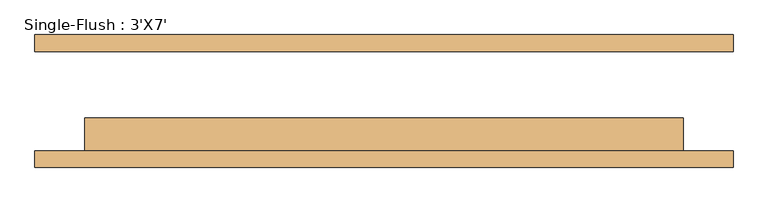
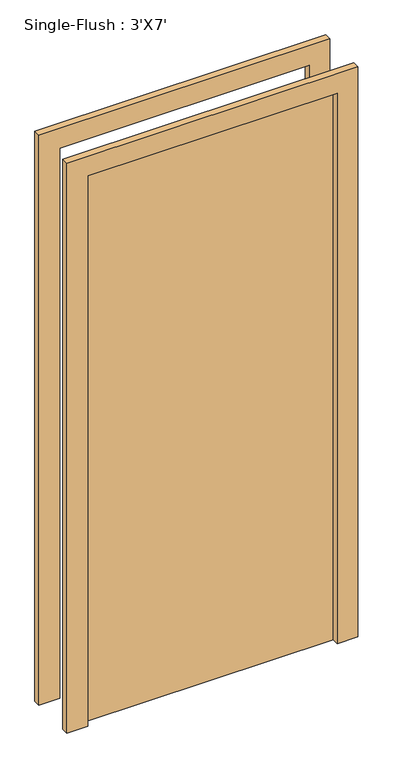
"""IFC4 building model written with IfcOpenShell, lengths in millimetres: door geometry, Single-Flush : 3'X7'."""

from ifc_helpers import new_model, si_unit, frame, origin, origin_with_axes, place, context, project, spatial, polyline, outline, extrude, source, transform, mapped, element, save


def single_flush_3_x7_686f89d2(model_context):
    return source(origin(), model_context, "Body", "SweptSolid", [
        extrude(outline(polyline([(2209.8, -533.4), (0.0, -533.4), (0.0, -457.2), (2133.6, -457.2), (2133.6, 457.2), (0.0, 457.2), (0.0, 533.4), (2209.8, 533.4), (2209.8, -533.4)])), frame((0.0, -101.6, 0.0), z_axis=(0.0, 1.0, 0.0), x_axis=(0.0, 0.0, 1.0)), (0.0, 0.0, 1.0), 25.4),
        extrude(outline(polyline([(2209.8, 533.4), (2209.8, -533.4), (0.0, -533.4), (0.0, -457.2), (2133.6, -457.2), (2133.6, 457.2), (0.0, 457.2), (0.0, 533.4), (2209.8, 533.4)])), frame((0.0, 76.2, 0.0), z_axis=(0.0, 1.0, 0.0), x_axis=(0.0, 0.0, 1.0)), (0.0, 0.0, 1.0), 25.4),
        extrude(outline(polyline([(457.2, -25.4), (457.2, -76.2), (-457.2, -76.2), (-457.2, -25.4), (457.2, -25.4)])), origin_with_axes(), (0.0, 0.0, 1.0), 2133.6),
    ])


if __name__ == "__main__":
    model = new_model("IFC4")
    model_context = context("Model", 3, world=origin())
    ifc_project = project(units=[si_unit("LENGTHUNIT", "METRE", prefix="MILLI")], contexts=[model_context])
    site = spatial("IfcSite", under=ifc_project)
    building = spatial("IfcBuilding", under=site)
    placement = place(None, origin())
    single_flush_3_x7_shape = single_flush_3_x7_686f89d2(model_context)
    element("IfcDoor", 1, ObjectType="Single-Flush : 3'X7'", at=placement, inside=building, context=model_context, shape_type="MappedRepresentation", body=[
        mapped(single_flush_3_x7_shape, transform((0.0, 0.0, 0.0), x_axis=(1.0, 0.0, 0.0), y_axis=(0.0, 1.0, 0.0), z_axis=(0.0, 0.0, 1.0))),
    ])
    save(model, "model.ifc")

# Revit data of these elements
# Type "Single-Flush : 3'X7'"
#   Type Mark = "8"
#   Construction Type Id = "MDOOR"
#   Assembly Code = "C1020"
#   Analytic Construction = "Metal"
#   Thickness = 0' - 2"
#   Heat Transfer Coefficient (U) = 0.651978 BTU/(h·ft²·°F)
#   Height = 7' - 0"
#   Trim Projection Ext = 0' - 1"
#   Trim Projection Int = 0' - 1"
#   Trim Width = 0' - 3"
#   Width = 3' - 0"
#   Define Thermal Properties by = 1
#   Door Material = Door - Panel
#   Frame Material = Door - Frame
#   Visual Light Transmittance = 0
#   Solar Heat Gain Coefficient = 0
#   Function = (empty or 0)
#   Wall Closure = (empty or 0)
# Element 1 (IfcDoor, "Single-Flush : 3'X7'")
#   Materials on its faces: "Door - Frame", "Door - Panel"
# Materials
#   "Door - Panel": class "Wood", colour RGB 210 159 95, transparency 0, Cost = 0
#   "Door - Frame": colour RGB 118 70 51, transparency 0, Cost = 0
